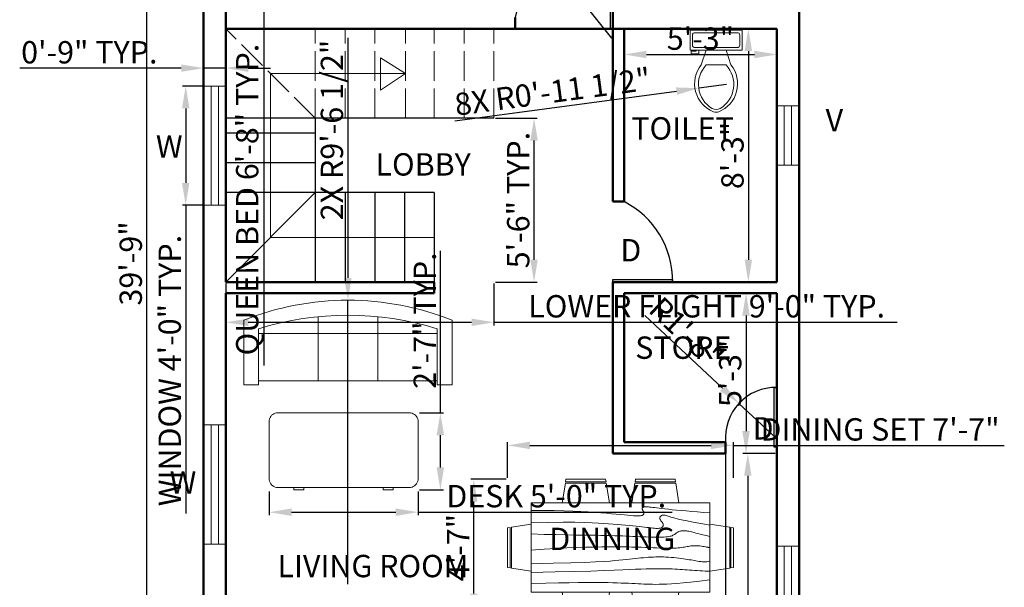
# Model space of a CAD drawing. Units: inches. Extents: x 1802 to 2621, y 1038 to 1686.
# Tile 2 of 5: x 1802 to 2198, y 1223 to 1452. Entities that reach past the tile are written whole.
import ezdxf

# ---------------------------------------------------------------- set-up
doc = ezdxf.new("R2010")
doc.units = ezdxf.units.IN
doc.linetypes.add('ACAD_ISO02W100', pattern=[15, 12, -3])
for name, color, linetype, lineweight in [('A-ANNO-DIMS', 2, 'Continuous', 18), ('A-ANNO-SYMB', 7, 'Continuous', 18), ('A-ANNO-TEXT', 7, 'Continuous', 18), ('A-AREA-IDEN', 7, 'Continuous', 25), ('A-DOOR', 3, 'Continuous', 25), ('A-FLOR-FIXT', 9, 'Continuous', 18), ('A-FLOR-STRS', 7, 'Continuous', 25), ('A-FLOR-STRS-OVHD', 8, 'ACAD_ISO02W100', 18), ('A-FURN', 8, 'Continuous', 18), ('A-GLAZ', 4, 'Continuous', 18), ('A-WALL', 7, 'Continuous', 50)]:
    doc.layers.add(name, color=color, linetype=linetype, lineweight=lineweight)
doc.styles.get("Standard").update_dxf_attribs({"font": 'arial.ttf'})
doc.dimstyles.new('ISO-25', dxfattribs={"dimtxt": 9, "dimasz": 9, "dimexe": 1.25, "dimexo": 0.625, "dimtad": 1, "dimdec": 1, "dimrnd": 9, "dimlunit": 3, "dimtxsty": 'Standard', "dimcen": 2.5, "dimadec": 0, "dimazin": 0, "dimtfac": 1, "dimtdec": 1, "dimtmove": 0, "dimatfit": 3, "dimfxl": 1, "dimarcsym": 0})

# ---------------------------------------------------------------- blocks, each defined once
blk = doc.blocks.new('*D4')
at = {"layer": 'A-ANNO-DIMS', "color": 0, "lineweight": -2, "transparency": 16777216}
for p, q in [((1875.1, 1593.56), (1851.51, 1593.56)), ((1852.76, 1584.56), (1852.76, 1122.56)), ((1875.1, 1113.56), (1851.51, 1113.56))]:
    blk.add_line(p, q, dxfattribs=at)
at = {"layer": 'A-ANNO-DIMS', "color": 0, "transparency": 16777216}
for points in [[(1851.26, 1584.56), (1854.26, 1584.56), (1852.76, 1593.56)], [(1851.26, 1122.56), (1854.26, 1122.56), (1852.76, 1113.56)]]:
    blk.add_solid(points, dxfattribs=at)
at = {"layer": 'Defpoints', "color": 0, "transparency": 16777216}
for p in [(1875.73, 1593.56), (1852.76, 1113.56), (1875.73, 1113.56)]:
    blk.add_point(p, dxfattribs=at)
at = {"layer": 'A-ANNO-DIMS', "color": 0, "transparency": 16777216, "insert": (1847.54, 1353.56), "char_height": 9, "attachment_point": 5, "rotation": 90}
blk.add_mtext('39\'-9"', dxfattribs=at)
blk = doc.blocks.new('*D6')
at = {"layer": 'A-ANNO-DIMS', "color": 0, "lineweight": -2, "transparency": 16777216}
for p, q in [((2106.1, 1448.06), (2094.04, 1448.06)), ((2095.29, 1439.06), (2095.29, 1355.06)), ((2106.1, 1346.06), (2094.04, 1346.06))]:
    blk.add_line(p, q, dxfattribs=at)
at = {"layer": 'A-ANNO-DIMS', "color": 0, "transparency": 16777216}
for points in [[(2093.79, 1439.06), (2096.79, 1439.06), (2095.29, 1448.06)], [(2093.79, 1355.06), (2096.79, 1355.06), (2095.29, 1346.06)]]:
    blk.add_solid(points, dxfattribs=at)
at = {"layer": 'Defpoints', "color": 0, "transparency": 16777216}
for p in [(2106.73, 1448.06), (2095.29, 1346.06), (2106.73, 1346.06)]:
    blk.add_point(p, dxfattribs=at)
at = {"layer": 'A-ANNO-DIMS', "color": 0, "transparency": 16777216, "insert": (2090.06, 1397.06), "char_height": 9, "attachment_point": 5, "rotation": 90}
blk.add_mtext('8\'-3"', dxfattribs=at)
blk = doc.blocks.new('*D7')
at = {"layer": 'A-ANNO-DIMS', "color": 0, "lineweight": -2, "transparency": 16777216}
for p, q in [((2106.1, 1341.56), (2093.11, 1341.56)), ((2094.36, 1332.56), (2094.36, 1286.06)), ((2106.1, 1277.06), (2093.11, 1277.06))]:
    blk.add_line(p, q, dxfattribs=at)
at = {"layer": 'A-ANNO-DIMS', "color": 0, "transparency": 16777216}
for points in [[(2092.86, 1332.56), (2095.86, 1332.56), (2094.36, 1341.56)], [(2092.86, 1286.06), (2095.86, 1286.06), (2094.36, 1277.06)]]:
    blk.add_solid(points, dxfattribs=at)
at = {"layer": 'Defpoints', "color": 0, "transparency": 16777216}
for p in [(2106.73, 1341.56), (2094.36, 1277.06), (2106.73, 1277.06)]:
    blk.add_point(p, dxfattribs=at)
at = {"layer": 'A-ANNO-DIMS', "color": 0, "transparency": 16777216, "insert": (2089.14, 1309.31), "char_height": 9, "attachment_point": 5, "rotation": 90}
blk.add_mtext('5\'-3"', dxfattribs=at)
blk = doc.blocks.new('*D8')
at = {"layer": 'A-ANNO-DIMS', "color": 0, "lineweight": -2, "transparency": 16777216}
for p, q in [((2106.1, 1277.06), (2093.83, 1277.06)), ((2095.08, 1268.06), (2095.08, 1131.56)), ((2106.1, 1122.56), (2093.83, 1122.56))]:
    blk.add_line(p, q, dxfattribs=at)
at = {"layer": 'A-ANNO-DIMS', "color": 0, "transparency": 16777216}
for points in [[(2093.58, 1268.06), (2096.58, 1268.06), (2095.08, 1277.06)], [(2093.58, 1131.56), (2096.58, 1131.56), (2095.08, 1122.56)]]:
    blk.add_solid(points, dxfattribs=at)
at = {"layer": 'Defpoints', "color": 0, "transparency": 16777216}
for p in [(2106.73, 1277.06), (2095.08, 1122.56), (2106.73, 1122.56)]:
    blk.add_point(p, dxfattribs=at)
at = {"layer": 'A-ANNO-DIMS', "color": 0, "transparency": 16777216, "insert": (2089.86, 1199.81), "char_height": 9, "attachment_point": 5, "rotation": 90}
blk.add_mtext('12\'-9"', dxfattribs=at)
blk = doc.blocks.new('*D11')
at = {"layer": 'A-ANNO-DIMS', "color": 0, "lineweight": -2, "transparency": 16777216}
for p, q in [((2045.23, 1447.43), (2045.23, 1436.45)), ((2106.73, 1447.43), (2106.73, 1436.45)), ((2054.23, 1437.7), (2097.73, 1437.7))]:
    blk.add_line(p, q, dxfattribs=at)
at = {"layer": 'A-ANNO-DIMS', "color": 0, "transparency": 16777216}
for points in [[(2054.23, 1439.2), (2054.23, 1436.2), (2045.23, 1437.7)], [(2097.73, 1439.2), (2097.73, 1436.2), (2106.73, 1437.7)]]:
    blk.add_solid(points, dxfattribs=at)
at = {"layer": 'Defpoints', "color": 0, "transparency": 16777216}
for p in [(2045.23, 1448.06), (2106.73, 1448.06), (2106.73, 1437.7)]:
    blk.add_point(p, dxfattribs=at)
at = {"layer": 'A-ANNO-DIMS', "color": 0, "transparency": 16777216, "insert": (2075.98, 1442.92), "char_height": 9, "attachment_point": 5}
blk.add_mtext('5\'-3"', dxfattribs=at)
blk = doc.blocks.new('Dining Set - 36 x 72 in.')
for p, q in [((-22.2343, 26.00059), (-23.4847, 17.99762)), ((-22.2304, 26), (-5.7608, 26)), ((-22, 27.5), (-22.1562, 26.50042)), ((-5.8416, 26.5), (-22.1534, 26.5)), ((-22, 27.5), (-6, 27.5)), ((-5.8437, 26.49966), (-6, 27.5)), ((-4.5152, 17.99762), (-5.7655, 25.99926)), ((5.7657, 26.00059), (4.5153, 17.99762)), ((5.7696, 26), (22.2392, 26)), ((6, 27.5), (5.8438, 26.50042)), ((22.1584, 26.5), (5.8466, 26.5)), ((6, 27.5), (22, 27.5)), ((22.1563, 26.49966), (22, 27.5)), ((23.4848, 17.99762), (22.2345, 25.99926)), ((36, 18), (-36, 18)), ((-36, 18), (-36, -18)), ((36, -18), (36, 18)), ((-45.5, 8), (-44.5004, 8.15617)), ((-45.5, 8), (-45.5, -8)), ((-44.5, -8.15843), (-44.5, 8.15338)), ((-44.0006, 8.23428), (-35.9976, 9.48474)), ((-44, 8.23041), (-44, -8.23915)), ((44.0006, 8.23428), (35.9976, 9.48474)), ((44, 8.23041), (44, -8.23915)), ((44.5, -8.15843), (44.5, 8.15338)), ((45.5, 8), (44.5005, 8.15617)), ((45.5, 8), (45.5, -8)), ((-44.4997, -8.15631), (-45.5, -8)), ((-35.9976, -9.48476), (-43.9993, -8.2345)), ((35.9976, -9.48476), (43.9993, -8.2345)), ((44.4997, -8.15631), (45.5, -8)), ((-36, -18), (36, -18)), ((-22.2343, -26.0006), (-23.4847, -17.99762)), ((-4.5152, -17.99762), (-5.7655, -25.99928)), ((5.7657, -26.0006), (4.5153, -17.99762)), ((23.4848, -17.99762), (22.2345, -25.99928)), ((-22.2304, -26), (-5.7608, -26)), ((-22, -27.5), (-22.1562, -26.50044)), ((-5.8416, -26.5), (-22.1534, -26.5)), ((-22, -27.5), (-6, -27.5)), ((-5.8437, -26.49967), (-6, -27.5)), ((5.7696, -26), (22.2392, -26)), ((6, -27.5), (5.8438, -26.50044)), ((22.1584, -26.5), (5.8466, -26.5)), ((6, -27.5), (22, -27.5)), ((22.1563, -26.49967), (22, -27.5))]:
    blk.add_line(p, q)
for points in [[(-36, 15), (-31.1772, 14.97754), (-26.8079, 14.91406), (-22.8538, 14.81543), (-19.276, 14.6875), (-16.0362, 14.53613), (-13.0957, 14.36718), (-10.4159, 14.18652), (-7.9583, 14), (-5.6904, 13.81315), (-3.6035, 13.63021), (-1.6954, 13.45508), (0.0365, 13.29166), (1.5945, 13.14388), (2.9811, 13.01562), (4.1988, 12.9108), (5.25, 12.83333), (6.1393, 12.78613), (6.8802, 12.76823), (7.4883, 12.77767), (7.9792, 12.8125), (8.3685, 12.87077), (8.6719, 12.95052), (8.9049, 13.0498), (9.0833, 13.16666), (9.2205, 13.29899), (9.3216, 13.44401), (9.3895, 13.59879), (9.4271, 13.76041), (9.4373, 13.92594), (9.4232, 14.09245), (9.3875, 14.257), (9.3333, 14.41666), (9.2638, 14.56917), (9.1836, 14.71484), (9.0975, 14.85465), (9.0104, 14.98958), (8.9272, 15.1206), (8.8529, 15.2487), (8.7922, 15.37483), (8.75, 15.5), (8.7305, 15.62467), (8.7344, 15.74739), (8.7617, 15.86621), (8.8125, 15.97916), (8.8867, 16.08431), (8.9844, 16.17968), (9.1055, 16.26334), (9.25, 16.33333), (9.4189, 16.38802), (9.6172, 16.42708), (9.8506, 16.45052), (10.125, 16.45833), (10.4463, 16.45052), (10.8203, 16.42708), (11.2529, 16.38802), (11.75, 16.33333), (12.3184, 16.26318), (12.9694, 16.17838), (13.7151, 16.07991), (14.5677, 15.96875), (15.5395, 15.84586), (16.6426, 15.71224), (17.8893, 15.56884), (19.2917, 15.41666), (20.859, 15.25667), (22.5879, 15.08984), (24.4721, 14.91715), (26.5052, 14.73958), (28.6809, 14.5581), (30.9929, 14.3737), (33.4347, 14.18733), (36, 14)], [(-36, 10), (-28.9766, 10.14274), (-23.1725, 10.20442), (-18.4241, 10.19775), (-14.5677, 10.13541), (-11.4399, 10.03011), (-8.877, 9.89453), (-6.7154, 9.74137), (-4.7917, 9.58333), (-2.9698, 9.43082), (-1.2246, 9.28515), (0.4415, 9.14534), (2.026, 9.01041), (3.5266, 8.87939), (4.9408, 8.7513), (6.266, 8.62516), (7.5, 8.5), (8.6411, 8.37549), (9.6914, 8.2539), (10.6538, 8.13818), (11.5312, 8.03125), (12.3267, 7.93603), (13.043, 7.85547), (13.6831, 7.79248), (14.25, 7.75), (14.7471, 7.7303), (15.1797, 7.73307), (15.5537, 7.75732), (15.875, 7.80208), (16.1494, 7.86637), (16.3828, 7.94922), (16.5811, 8.04964), (16.75, 8.16666), (16.8944, 8.29915), (17.0143, 8.44531), (17.1089, 8.60319), (17.1771, 8.77083), (17.218, 8.94629), (17.2305, 9.1276), (17.2137, 9.31282), (17.1667, 9.5), (17.0895, 9.6875), (16.987, 9.875), (16.8649, 10.0625), (16.7292, 10.25), (16.5856, 10.4375), (16.4401, 10.625), (16.2985, 10.8125), (16.1667, 11), (16.05, 11.18733), (15.9518, 11.3737), (15.8752, 11.5581), (15.8229, 11.73958), (15.798, 11.91715), (15.8034, 12.08984), (15.842, 12.25667), (15.9167, 12.41666), (16.0295, 12.56836), (16.1784, 12.70833), (16.3605, 12.83268), (16.5729, 12.9375), (16.8127, 13.01888), (17.0768, 13.07291), (17.3625, 13.0957), (17.6667, 13.08333), (17.9894, 13.03312), (18.3418, 12.94726), (18.7382, 12.82918), (19.1927, 12.68229), (19.7195, 12.51001), (20.3327, 12.31575), (21.0465, 12.10294), (21.875, 11.875), (22.8357, 11.63354), (23.959, 11.37304), (25.2786, 11.08618), (26.8282, 10.76562), (28.6414, 10.40405), (30.752, 9.99414), (33.1936, 9.52856), (36, 9)], [(-36, 5.5), (-30.7157, 5.3348), (-26.069, 5.20963), (-21.9946, 5.11767), (-18.4271, 5.05208), (-15.3009, 5.00602), (-12.5508, 4.97265), (-10.1112, 4.94515), (-7.9167, 4.91666), (-5.909, 4.88167), (-4.0586, 4.83984), (-2.3429, 4.79215), (-0.7396, 4.73958), (0.7739, 4.6831), (2.22, 4.6237), (3.6213, 4.56233), (5, 4.5), (6.373, 4.43782), (7.7344, 4.3776), (9.0723, 4.32129), (10.375, 4.27083), (11.6309, 4.22819), (12.8281, 4.19531), (13.9551, 4.17415), (15, 4.16666), (15.954, 4.17448), (16.819, 4.19791), (17.6001, 4.23698), (18.3021, 4.29166), (18.9299, 4.36198), (19.4883, 4.44791), (19.9823, 4.54948), (20.4167, 4.66666), (20.7969, 4.79899), (21.1302, 4.94401), (21.4245, 5.09879), (21.6875, 5.26041), (21.9271, 5.42594), (22.1511, 5.59245), (22.3672, 5.757), (22.5834, 5.91666), (22.8065, 6.06868), (23.0404, 6.21093), (23.2879, 6.34147), (23.5521, 6.45833), (23.8358, 6.55957), (24.142, 6.64323), (24.4735, 6.70735), (24.8334, 6.75), (25.2235, 6.76969), (25.642, 6.76692), (26.0858, 6.74267), (26.5521, 6.69791), (27.0379, 6.63362), (27.5404, 6.55078), (28.0565, 6.45036), (28.5834, 6.33333), (29.1242, 6.19987), (29.7071, 6.04687), (30.3661, 5.87044), (31.1354, 5.66666), (32.0493, 5.43164), (33.142, 5.16146), (34.4475, 4.85221), (36, 4.5)], [(-36, -1), (-30.7915, -0.6591), (-26.0195, -0.38216), (-21.6519, -0.16284), (-17.6563, 0.00521), (-14.0005, 0.12833), (-10.6523, 0.21289), (-7.5796, 0.26522), (-4.75, 0.29166), (-2.134, 0.29793), (0.2878, 0.28711), (2.5317, 0.26163), (4.6146, 0.22396), (6.5529, 0.17651), (8.3633, 0.12174), (10.0623, 0.06209), (11.6667, 0), (13.1899, -0.06201), (14.6341, -0.1211), (15.9982, -0.17432), (17.2813, -0.21875), (18.4823, -0.25147), (19.6003, -0.26953), (20.6343, -0.27002), (21.5834, -0.25), (22.4481, -0.20768), (23.2357, -0.14584), (23.9549, -0.06836), (24.6146, 0.02083), (25.2235, 0.11784), (25.7904, 0.21875), (26.3241, 0.31966), (26.8334, 0.41666), (27.3265, 0.50618), (27.8099, 0.58593), (28.2894, 0.65397), (28.7709, 0.70833), (29.2601, 0.74707), (29.763, 0.76823), (30.2855, 0.76985), (30.8334, 0.75), (31.4088, 0.70784), (31.9994, 0.64713), (32.589, 0.57275), (33.1615, 0.48958), (33.7008, 0.4025), (34.1908, 0.3164), (34.6153, 0.23616), (34.9584, 0.16666), (35.2099, 0.11165), (35.3848, 0.07031), (35.504, 0.04069), (35.5886, 0.02083), (35.6594, 0.00879), (35.7377, 0.0026), (35.8442, 0.00032), (36, 0)], [(-36, -6.5), (-27.1843, -6.31267), (-20.084, -6.1263), (-14.469, -5.9419), (-10.1094, -5.76042), (-6.7752, -5.58285), (-4.2363, -5.41016), (-2.2629, -5.24333), (-0.625, -5.08334), (0.8708, -4.93099), (2.2715, -4.78646), (3.5872, -4.64974), (4.8281, -4.52084), (6.0046, -4.39974), (7.127, -4.28646), (8.2053, -4.18099), (9.25, -4.08334), (10.2705, -3.99382), (11.2734, -3.91407), (12.2647, -3.84603), (13.25, -3.79167), (14.2354, -3.75293), (15.2266, -3.73177), (16.2295, -3.73015), (17.25, -3.75), (18.2912, -3.79248), (19.3451, -3.85547), (20.4009, -3.93604), (21.4479, -4.03125), (22.4754, -4.13819), (23.4727, -4.25391), (24.4289, -4.37549), (25.3334, -4.5), (26.1785, -4.62492), (26.9694, -4.74935), (27.7145, -4.87281), (28.4219, -4.99479), (29.1, -5.11483), (29.7572, -5.23242), (30.4016, -5.34709), (31.0417, -5.45834), (31.6837, -5.56437), (32.3262, -5.65821), (32.9658, -5.73153), (33.599, -5.77604), (34.2224, -5.78345), (34.8327, -5.74545), (35.4264, -5.65373), (36, -5.5)], [(-36, -10), (-26.4022, -9.81299), (-18.4675, -9.62891), (-11.9839, -9.45069), (-6.7396, -9.28125), (-2.5226, -9.12354), (0.8789, -8.98047), (3.6769, -8.85498), (6.0833, -8.75), (8.2767, -8.66765), (10.3021, -8.60677), (12.1712, -8.56543), (13.8958, -8.54167), (15.4876, -8.53353), (16.9583, -8.53907), (18.3197, -8.55632), (19.5834, -8.58334), (20.7616, -8.61841), (21.8685, -8.66081), (22.9188, -8.71004), (23.9271, -8.76563), (24.9081, -8.82707), (25.8763, -8.89388), (26.8465, -8.96558), (27.8334, -9.04167), (28.8474, -9.12118), (29.8828, -9.20117), (30.93, -9.27824), (31.9792, -9.34896), (33.0205, -9.40991), (34.0443, -9.45768), (35.0407, -9.48885), (36, -9.5)], [(-36, -14.5), (-30.0881, -14.33513), (-25.0332, -14.21224), (-20.7312, -14.12647), (-17.0781, -14.07292), (-13.97, -14.04671), (-11.3027, -14.04297), (-8.9724, -14.05681), (-6.875, -14.08334), (-4.9224, -14.11833), (-3.0905, -14.16016), (-1.3709, -14.20785), (0.2448, -14.26042), (1.7647, -14.3169), (3.1973, -14.3763), (4.5507, -14.43767), (5.8333, -14.5), (7.0554, -14.5621), (8.235, -14.62175), (9.3922, -14.67652), (10.5469, -14.72396), (11.7192, -14.76164), (12.929, -14.78711), (14.1965, -14.79794), (15.5417, -14.79167), (16.9933, -14.76424), (18.6152, -14.70508), (20.4804, -14.60197), (22.6615, -14.44271), (25.2312, -14.21509), (28.2624, -13.9069), (31.8277, -13.50594), (36, -13)]]:
    blk.add_lwpolyline(points)
blk = doc.blocks.new('Toilet - top')
for p, q in [((9.5, -6), (9.5, -2)), ((-10, -8.5), (-8, -8.5)), ((-10, -9.5), (-10, -8.5)), ((-7, -9.5), (-10, -9.5)), ((-8, -8.5), (-8, -8)), ((-7, -8), (-7, -9.5)), ((-4, -8), (-6, -14)), ((4, -8), (6, -14)), ((4, -14), (-4, -14))]:
    blk.add_line(p, q)
blk.add_lwpolyline([(10.5, -8), (10.5, 0), (-10.5, 0), (-10.5, -8)], close=True)
for points in [[(-9.5, -2), (-9.5, -6)], [(8.5, -1), (-8.5, -1)], [(-8.5, -7), (8.5, -7)]]:
    blk.add_lwpolyline(points)
for centre, radius, start, end in [((-8.62, -1.88), 0.884, 81.8699, 188.1301), ((8.62, -1.88), 0.884, 351.8699, 98.1301), ((-8.62, -6.12), 0.884, 171.8699, 278.1301), ((8.62, -6.12), 0.884, 261.8699, 8.1301), ((3.52, -21.58), 12.17, 141.4691, 247.9714), ((4.2, -21.82), 11.33, 136.3677, 238.9468), ((-3.52, -21.58), 12.17, 292.0284, 38.5307), ((-4.2, -21.82), 11.33, 301.053, 43.6321), ((0, -27.88), 4, 245.7318, 294.2682), ((0, -29), 4, 254.8605, 285.1395)]:
    blk.add_arc(centre, radius, start, end)
blk = doc.blocks.new('Sofa - Roundback 7 ft.')
for p, q in [((-12.00002, -32.4421), (-12.00003, -6.5971)), ((11.99997, -32.4421), (11.99998, -6.5971)), ((-36.000027, -34), (-36.000027, -11.4696)), ((35.99998, -34), (35.99998, -11.4696)), ((-35.999844, -13.3819), (35.9998, -13.3819)), ((-36.000027, -32.4421), (35.99998, -32.4421))]:
    blk.add_line(p, q)
for points in [[(-36.000027, -34), (-42.000027, -34), (-42.000027, -8)], [(41.99998, -8), (41.99998, -34), (35.99998, -34)]]:
    blk.add_lwpolyline(points)
for centre, radius, start, end in [((0, -114.25), 114.25, 68.43141, 111.5686), ((-0.00001, -127.1968), 121.1968, 72.72033, 107.2797)]:
    blk.add_arc(centre, radius, start, end)
blk = doc.blocks.new('Desk - 30 x 60 in.')
for p, q in [((-26.999995, 0), (26.999995, 0)), ((-29.999995, -27), (-29.999995, -3)), ((29.999995, -3), (29.999995, -27)), ((26.999995, -30), (-26.999995, -30)), ((-20.000005, -30), (-20.000005, -31)), ((-20.000005, -31), (-16.000005, -31)), ((-16.000005, -31), (-16.000005, -30)), ((15.999995, -31), (15.999995, -30)), ((19.999995, -31), (15.999995, -31)), ((19.999995, -30), (19.999995, -31))]:
    blk.add_line(p, q)
for centre, start, end in [((-26.499995, -3.5), 98.1301, 171.8699), ((26.499995, -3.5), 8.130102, 81.8699), ((-26.499995, -26.5), 188.1301, 261.8699), ((26.499995, -26.5), 278.1301, 351.8699)]:
    blk.add_arc(centre, 3.535534, start, end)
blk = doc.blocks.new('WIN-48IN')
for p, q in [((9, 48), (0, 48)), ((3, 48), (3, 0)), ((6, 48), (6, 0)), ((9, 0), (0, 0))]:
    blk.add_line(p, q)
blk = doc.blocks.new('VENT-24IN')
for p, q in [((0, 24), (9, 24)), ((3, 0), (3, 24)), ((6, 0), (6, 24)), ((0, 0), (9, 0))]:
    blk.add_line(p, q)
blk = doc.blocks.new('DOOR-BEDROOM-36IN')
for p, q in [((38.47, 0), (38.47, 36)), ((38.47, 36), (39.47, 36)), ((39.47, 0), (38.47, 0))]:
    blk.add_line(p, q)
blk.add_arc((38.97, -3.86), 39.86, 89.2813, 167.8967)
blk = doc.blocks.new('DOOR-BATH-LOBBY-24IN')
for p, q in [((0, 0), (0, 1)), ((0, 1), (24, 1)), ((24, 1), (24, 0))]:
    blk.add_line(p, q)
blk.add_arc((-11.84, 0.5), 35.84, 359.2007, 62.8783)
blk = doc.blocks.new('STAIR-DIRECTION-U')
for p, q in [((44.37, 59.29), (44.37, 72.31)), ((44.37, 72.31), (54.34, 66)), ((0, 0), (0, 66)), ((0, 66), (54.34, 66)), ((54.34, 66), (44.37, 59.29)), ((66, 0), (0, 0))]:
    blk.add_line(p, q)
blk = doc.blocks.new('STAIR-WINDER-UPPER-TREADS')
for p, q in [((36, 0), (0, 36)), ((36, 0), (36, 36)), ((48, 0), (48, 36)), ((60, 0), (60, 36)), ((72.34, 0), (72.34, 36)), ((84, 0), (84, 36)), ((96, 0), (96, 36)), ((108, 0), (108, 36))]:
    blk.add_line(p, q)
blk = doc.blocks.new('STAIR-WINDER-VISIBLE')
for p, q in [((108, 66), (0, 66)), ((36, 66), (36, 0)), ((36, 60), (0, 60)), ((36, 48), (0, 48)), ((84, 36), (0, 36)), ((36, 36), (0, 0)), ((48, 36), (48, 0)), ((60, 36), (60, 0)), ((72, 36), (72, 0)), ((84, 36), (84, 0))]:
    blk.add_line(p, q)
blk = doc.blocks.new('*D37')
at = {"layer": 'A-ANNO-DIMS', "color": 0, "lineweight": -2, "transparency": 16777216}
for p, q in [((1875.1, 1425), (1867.28, 1425)), ((1868.53, 1416), (1868.53, 1386)), ((1875.1, 1377), (1867.28, 1377)), ((1868.53, 1377), (1868.53, 1252.86))]:
    blk.add_line(p, q, dxfattribs=at)
at = {"layer": 'A-ANNO-DIMS', "color": 0, "transparency": 16777216}
for points in [[(1867.03, 1416), (1870.03, 1416), (1868.53, 1425)], [(1867.03, 1386), (1870.03, 1386), (1868.53, 1377)]]:
    blk.add_solid(points, dxfattribs=at)
at = {"layer": 'Defpoints', "color": 0, "transparency": 16777216}
for p in [(1875.73, 1425), (1868.53, 1377), (1875.73, 1377)]:
    blk.add_point(p, dxfattribs=at)
at = {"layer": 'A-ANNO-DIMS', "color": 0, "transparency": 16777216, "insert": (1863.25, 1310.43), "char_height": 9, "attachment_point": 5, "rotation": 90}
blk.add_mtext('WINDOW 4\'-0" TYP.', dxfattribs=at)
blk = doc.blocks.new('*D38')
at = {"layer": 'A-ANNO-DIMS', "color": 0, "lineweight": -2, "transparency": 16777216}
for p, q in [((1875.73, 1425.62), (1875.73, 1433.45)), ((1884.73, 1425.62), (1884.73, 1433.45)), ((1866.73, 1432.2), (1801.62, 1432.2)), ((1884.73, 1432.2), (1875.73, 1432.2)), ((1893.73, 1432.2), (1902.73, 1432.2))]:
    blk.add_line(p, q, dxfattribs=at)
at = {"layer": 'A-ANNO-DIMS', "color": 0, "transparency": 16777216}
for points in [[(1866.73, 1433.7), (1866.73, 1430.7), (1875.73, 1432.2)], [(1893.73, 1433.7), (1893.73, 1430.7), (1884.73, 1432.2)]]:
    blk.add_solid(points, dxfattribs=at)
at = {"layer": 'Defpoints', "color": 0, "transparency": 16777216}
for p in [(1875.73, 1432.2), (1875.73, 1425), (1884.73, 1425)]:
    blk.add_point(p, dxfattribs=at)
at = {"layer": 'A-ANNO-DIMS', "color": 0, "transparency": 16777216, "insert": (1829.68, 1437.42), "char_height": 9, "attachment_point": 5}
blk.add_mtext('0\'-9" TYP.', dxfattribs=at)
blk = doc.blocks.new('*D43')
at = {"layer": 'A-ANNO-DIMS', "color": 0, "lineweight": -2, "transparency": 16777216}
for p, q in [((1911.42, 1535.09), (1898.79, 1535.09)), ((1900.04, 1526.09), (1900.04, 1464.09)), ((1911.42, 1455.09), (1898.79, 1455.09)), ((1900.04, 1455.09), (1900.04, 1312.45))]:
    blk.add_line(p, q, dxfattribs=at)
at = {"layer": 'A-ANNO-DIMS', "color": 0, "transparency": 16777216}
for points in [[(1898.54, 1526.09), (1901.54, 1526.09), (1900.04, 1535.09)], [(1898.54, 1464.09), (1901.54, 1464.09), (1900.04, 1455.09)]]:
    blk.add_solid(points, dxfattribs=at)
at = {"layer": 'Defpoints', "color": 0, "transparency": 16777216}
for p in [(1912.04, 1535.09), (1900.04, 1455.09), (1912.04, 1455.09)]:
    blk.add_point(p, dxfattribs=at)
at = {"layer": 'A-ANNO-DIMS', "color": 0, "transparency": 16777216, "insert": (1894.49, 1379.27), "char_height": 9, "attachment_point": 5, "rotation": 90}
blk.add_mtext('QUEEN BED 6\'-8" TYP.', dxfattribs=at)
blk = doc.blocks.new('*D47')
at = {"layer": 'A-ANNO-DIMS', "color": 0, "lineweight": -2, "transparency": 16777216}
for p, q in [((1902.17, 1261.78), (1902.17, 1252.16)), ((1962.17, 1261.78), (1962.17, 1252.16)), ((1911.17, 1253.41), (1953.17, 1253.41)), ((1962.17, 1253.41), (2064.56, 1253.41))]:
    blk.add_line(p, q, dxfattribs=at)
at = {"layer": 'A-ANNO-DIMS', "color": 0, "transparency": 16777216}
for points in [[(1911.17, 1254.91), (1911.17, 1251.91), (1902.17, 1253.41)], [(1953.17, 1254.91), (1953.17, 1251.91), (1962.17, 1253.41)]]:
    blk.add_solid(points, dxfattribs=at)
at = {"layer": 'Defpoints', "color": 0, "transparency": 16777216}
for p in [(1902.17, 1262.41), (1962.17, 1262.41), (1962.17, 1253.41)]:
    blk.add_point(p, dxfattribs=at)
at = {"layer": 'A-ANNO-DIMS', "color": 0, "transparency": 16777216, "insert": (2017.87, 1258.69), "char_height": 9, "attachment_point": 5}
blk.add_mtext('DESK 5\'-0" TYP.', dxfattribs=at)
blk = doc.blocks.new('*D48')
at = {"layer": 'A-ANNO-DIMS', "color": 0, "lineweight": -2, "transparency": 16777216}
for p, q in [((1971.17, 1293.41), (1971.17, 1358.67)), ((1962.8, 1293.41), (1972.42, 1293.41)), ((1971.17, 1271.41), (1971.17, 1284.41)), ((1962.8, 1262.41), (1972.42, 1262.41))]:
    blk.add_line(p, q, dxfattribs=at)
at = {"layer": 'A-ANNO-DIMS', "color": 0, "transparency": 16777216}
for points in [[(1969.67, 1284.41), (1972.67, 1284.41), (1971.17, 1293.41)], [(1969.67, 1271.41), (1972.67, 1271.41), (1971.17, 1262.41)]]:
    blk.add_solid(points, dxfattribs=at)
at = {"layer": 'Defpoints', "color": 0, "transparency": 16777216}
for p in [(1962.17, 1293.41), (1971.17, 1293.41), (1962.17, 1262.41)]:
    blk.add_point(p, dxfattribs=at)
at = {"layer": 'A-ANNO-DIMS', "color": 0, "transparency": 16777216, "insert": (1966.03, 1330.54), "char_height": 9, "attachment_point": 5, "rotation": 90}
blk.add_mtext('2\'-7" TYP.', dxfattribs=at)
blk = doc.blocks.new('*D55')
at = {"layer": 'A-ANNO-DIMS', "color": 0, "lineweight": -2, "transparency": 16777216}
for p, q in [((1884.73, 1345.43), (1884.73, 1328.61)), ((1992.73, 1345.43), (1992.73, 1328.61)), ((1893.73, 1329.86), (1983.73, 1329.86)), ((1992.73, 1329.86), (2155.24, 1329.86))]:
    blk.add_line(p, q, dxfattribs=at)
at = {"layer": 'A-ANNO-DIMS', "color": 0, "transparency": 16777216}
for points in [[(1893.73, 1331.36), (1893.73, 1328.36), (1884.73, 1329.86)], [(1983.73, 1331.36), (1983.73, 1328.36), (1992.73, 1329.86)]]:
    blk.add_solid(points, dxfattribs=at)
at = {"layer": 'Defpoints', "color": 0, "transparency": 16777216}
for p in [(1884.73, 1346.06), (1992.73, 1346.06), (1992.73, 1329.86)]:
    blk.add_point(p, dxfattribs=at)
at = {"layer": 'A-ANNO-DIMS', "color": 0, "transparency": 16777216, "insert": (2078.48, 1335.14), "char_height": 9, "attachment_point": 5}
blk.add_mtext('LOWER FLIGHT 9\'-0" TYP.', dxfattribs=at)
blk = doc.blocks.new('*D56')
at = {"layer": 'A-ANNO-DIMS', "color": 0, "lineweight": -2, "transparency": 16777216}
for p, q in [((1993.35, 1412.06), (2010.18, 1412.06)), ((2008.93, 1355.06), (2008.93, 1403.06)), ((1993.35, 1346.06), (2010.18, 1346.06))]:
    blk.add_line(p, q, dxfattribs=at)
at = {"layer": 'A-ANNO-DIMS', "color": 0, "transparency": 16777216}
for points in [[(2007.43, 1403.06), (2010.43, 1403.06), (2008.93, 1412.06)], [(2007.43, 1355.06), (2010.43, 1355.06), (2008.93, 1346.06)]]:
    blk.add_solid(points, dxfattribs=at)
at = {"layer": 'Defpoints', "color": 0, "transparency": 16777216}
for p in [(1992.73, 1412.06), (2008.93, 1412.06), (1992.73, 1346.06)]:
    blk.add_point(p, dxfattribs=at)
at = {"layer": 'A-ANNO-DIMS', "color": 0, "transparency": 16777216, "insert": (2003.71, 1379.06), "char_height": 9, "attachment_point": 5, "rotation": 90}
blk.add_mtext('5\'-6" TYP.', dxfattribs=at)
blk = doc.blocks.new('*D59')
at = {"layer": 'A-ANNO-DIMS', "color": 0, "lineweight": -2, "transparency": 16777216}
for p, q in [((1998.28, 1267.27), (1998.28, 1281.55)), ((2007.28, 1280.3), (2080.28, 1280.3)), ((2089.28, 1267.27), (2089.28, 1281.55)), ((2089.28, 1280.3), (2198.45, 1280.3))]:
    blk.add_line(p, q, dxfattribs=at)
at = {"layer": 'A-ANNO-DIMS', "color": 0, "transparency": 16777216}
for points in [[(2007.28, 1281.8), (2007.28, 1278.8), (1998.28, 1280.3)], [(2080.28, 1281.8), (2080.28, 1278.8), (2089.28, 1280.3)]]:
    blk.add_solid(points, dxfattribs=at)
at = {"layer": 'Defpoints', "color": 0, "transparency": 16777216}
for p in [(2089.28, 1280.3), (1998.28, 1266.65), (2089.28, 1266.65)]:
    blk.add_point(p, dxfattribs=at)
at = {"layer": 'A-ANNO-DIMS', "color": 0, "transparency": 16777216, "insert": (2148.37, 1285.58), "char_height": 9, "attachment_point": 5}
blk.add_mtext('DINING SET 7\'-7"', dxfattribs=at)
blk = doc.blocks.new('*D60')
at = {"layer": 'A-ANNO-DIMS', "color": 0, "lineweight": -2, "transparency": 16777216}
for p, q in [((1997.66, 1266.65), (1983.38, 1266.65)), ((1984.63, 1220.65), (1984.63, 1257.65)), ((1997.66, 1211.65), (1983.38, 1211.65))]:
    blk.add_line(p, q, dxfattribs=at)
at = {"layer": 'A-ANNO-DIMS', "color": 0, "transparency": 16777216}
for points in [[(1983.13, 1257.65), (1986.13, 1257.65), (1984.63, 1266.65)], [(1983.13, 1220.65), (1986.13, 1220.65), (1984.63, 1211.65)]]:
    blk.add_solid(points, dxfattribs=at)
at = {"layer": 'Defpoints', "color": 0, "transparency": 16777216}
for p in [(1984.63, 1266.65), (1998.28, 1266.65), (1998.28, 1211.65)]:
    blk.add_point(p, dxfattribs=at)
at = {"layer": 'A-ANNO-DIMS', "color": 0, "transparency": 16777216, "insert": (1979.51, 1239.15), "char_height": 9, "attachment_point": 5, "rotation": 90}
blk.add_mtext('4\'-7"', dxfattribs=at)
blk = doc.blocks.new('*D75')
at = {"layer": 'A-ANNO-DIMS', "color": 0, "lineweight": -2, "transparency": 16777216}
for p, q in [((2086.14, 1280.93), (2086.14, 1082.61)), ((2106.73, 1278.98), (2106.73, 1082.61)), ((2095.14, 1083.86), (2097.73, 1083.86)), ((2106.73, 1083.86), (2161.03, 1083.86))]:
    blk.add_line(p, q, dxfattribs=at)
at = {"layer": 'A-ANNO-DIMS', "color": 0, "transparency": 16777216}
for points in [[(2095.14, 1085.36), (2095.14, 1082.36), (2086.14, 1083.86)], [(2097.73, 1085.36), (2097.73, 1082.36), (2106.73, 1083.86)]]:
    blk.add_solid(points, dxfattribs=at)
at = {"layer": 'Defpoints', "color": 0, "transparency": 16777216}
for p in [(2086.14, 1281.56), (2106.73, 1279.61), (2106.73, 1083.86)]:
    blk.add_point(p, dxfattribs=at)
at = {"layer": 'A-ANNO-DIMS', "color": 0, "transparency": 16777216, "insert": (2138.38, 1089.14), "char_height": 9, "attachment_point": 5}
blk.add_mtext('1\'-8 1/2"', dxfattribs=at)
blk = doc.blocks.new('*D79')
at = {"layer": 'A-ANNO-DIMS', "color": 0, "lineweight": -2, "transparency": 16777216}
for p, q in [((2053.63, 1332.55), (2084.91, 1303.35)), ((2106.23, 1283.44), (2091.48, 1297.21))]:
    blk.add_line(p, q, dxfattribs=at)
at = {"layer": 'A-ANNO-DIMS', "color": 0, "transparency": 16777216}
blk.add_solid([(2085.93, 1304.44), (2083.88, 1302.25), (2091.48, 1297.21)], dxfattribs=at)
at = {"layer": 'Defpoints', "color": 0, "transparency": 16777216}
for p in [(2091.48, 1297.21), (2106.23, 1283.44)]:
    blk.add_point(p, dxfattribs=at)
at = {"layer": 'A-ANNO-DIMS', "color": 0, "transparency": 16777216, "insert": (2069.54, 1324.84), "char_height": 9, "attachment_point": 5, "rotation": 316.9628}
blk.add_mtext('R1\'-8"', dxfattribs=at)
blk = doc.blocks.new('*D81')
at = {"layer": 'A-ANNO-DIMS', "color": 0, "lineweight": -2, "transparency": 16777216}
for p, q in [((1970.91, 1531.07), (2009.75, 1482.39)), ((2040.23, 1444.2), (2015.37, 1475.36))]:
    blk.add_line(p, q, dxfattribs=at)
at = {"layer": 'A-ANNO-DIMS', "color": 0, "transparency": 16777216}
blk.add_solid([(2010.93, 1483.33), (2008.58, 1481.46), (2015.37, 1475.36)], dxfattribs=at)
at = {"layer": 'Defpoints', "color": 0, "transparency": 16777216}
for p in [(2015.37, 1475.36), (2040.23, 1444.2)]:
    blk.add_point(p, dxfattribs=at)
at = {"layer": 'A-ANNO-DIMS', "color": 0, "transparency": 16777216, "insert": (1991.61, 1513.51), "char_height": 9, "attachment_point": 5, "rotation": 308.5892}
blk.add_mtext('2X R3\'-4"', dxfattribs=at)
blk = doc.blocks.new('*D85')
at = {"layer": 'A-ANNO-DIMS', "color": 0, "lineweight": -2, "transparency": 16777216}
for p, q in [((1933.91, 1444.41), (1933.91, 1347.74)), ((1933.91, 1224.49), (1933.91, 1338.74))]:
    blk.add_line(p, q, dxfattribs=at)
at = {"layer": 'A-ANNO-DIMS', "color": 0, "transparency": 16777216}
blk.add_solid([(1932.41, 1347.74), (1935.41, 1347.74), (1933.91, 1338.74)], dxfattribs=at)
at = {"layer": 'Defpoints', "color": 0, "transparency": 16777216}
for p in [(1933.91, 1338.74), (1933.91, 1224.49)]:
    blk.add_point(p, dxfattribs=at)
at = {"layer": 'A-ANNO-DIMS', "color": 0, "transparency": 16777216, "insert": (1928.63, 1407.29), "char_height": 9, "attachment_point": 5, "rotation": 89.9998}
blk.add_mtext('2X R9\'-6 1/2"', dxfattribs=at)
blk = doc.blocks.new('*D87')
at = {"layer": 'A-ANNO-DIMS', "color": 0, "lineweight": -2, "transparency": 16777216}
for p, q in [((2086.5, 1425.65), (2075.27, 1424.14)), ((1977.05, 1410.94), (2066.35, 1422.95))]:
    blk.add_line(p, q, dxfattribs=at)
at = {"layer": 'A-ANNO-DIMS', "color": 0, "transparency": 16777216}
blk.add_solid([(2066.15, 1424.43), (2066.55, 1421.46), (2075.27, 1424.14)], dxfattribs=at)
at = {"layer": 'Defpoints', "color": 0, "transparency": 16777216}
for p in [(2086.5, 1425.65), (2075.27, 1424.14)]:
    blk.add_point(p, dxfattribs=at)
at = {"layer": 'A-ANNO-DIMS', "color": 0, "transparency": 16777216, "insert": (2016.54, 1421.58), "char_height": 9, "attachment_point": 5, "rotation": 7.6552}
blk.add_mtext('8X R0\'-11 1/2"', dxfattribs=at)

msp = doc.modelspace()

# ---------------------------------------------------------------- linework, layer by layer
at = {"layer": 'A-DOOR'}
for p, q in [((2105.73, 1279.61), (2105.73, 1303.61)), ((2105.73, 1303.61), (2106.73, 1303.61)), ((2106.73, 1279.61), (2105.73, 1279.61))]:
    msp.add_line(p, q, dxfattribs=at)
msp.add_arc((2106.23, 1283.44), 20.18, 88.5799, 185.3459, dxfattribs=at)
at = {"layer": 'A-WALL'}
for p, q in [((1875.73, 1593.56), (1875.73, 1113.56)), ((2115.73, 1113.56), (2115.73, 1593.56)), ((1884.73, 1584.56), (1884.73, 1346.06)), ((2040.73, 1560.96), (2040.73, 1378.46)), ((2001.26, 1452.56), (2001.26, 1448.06)), ((2106.73, 1448.06), (1884.73, 1448.06)), ((2045.23, 1448.06), (2045.23, 1378.46)), ((2106.73, 1346.06), (2106.73, 1448.06)), ((2045.23, 1378.46), (2040.73, 1378.46)), ((1968.73, 1346.06), (1884.73, 1346.06)), ((1968.73, 1346.06), (1968.73, 1341.56)), ((2106.73, 1346.06), (2040.73, 1346.06)), ((2040.73, 1346.06), (2040.73, 1277.06)), ((1884.73, 1341.56), (1884.73, 1122.56)), ((1968.73, 1341.56), (1884.73, 1341.56)), ((2106.73, 1341.56), (2045.23, 1341.56)), ((2045.23, 1341.56), (2045.23, 1281.56)), ((2106.73, 1122.56), (2106.73, 1341.56)), ((2086.14, 1281.56), (2045.23, 1281.56)), ((2086.14, 1281.56), (2086.14, 1277.06)), ((2086.14, 1277.06), (2040.73, 1277.06))]:
    msp.add_line(p, q, dxfattribs=at)

# ---------------------------------------------------------------- block references
at = {"layer": 'A-ANNO-SYMB'}
msp.add_blockref('STAIR-DIRECTION-U', (1902.73, 1364.06), dxfattribs=at)
at = {"layer": 'A-DOOR'}
for name, p in [('DOOR-BEDROOM-36IN', (2001.26, 1448.06)), ('DOOR-BATH-LOBBY-24IN', (2040.73, 1346.06))]:
    msp.add_blockref(name, p, dxfattribs=at)
at = {"layer": 'A-FLOR-FIXT'}
msp.add_blockref('Toilet - top', (2082.3, 1447.47), dxfattribs=at)
at = {"layer": 'A-FLOR-STRS'}
msp.add_blockref('STAIR-WINDER-VISIBLE', (1884.73, 1346.06), dxfattribs=at)
at = {"layer": 'A-FLOR-STRS-OVHD'}
msp.add_blockref('STAIR-WINDER-UPPER-TREADS', (1884.73, 1412.06), dxfattribs=at)
at = {"layer": 'A-FURN'}
for name, p in [('Sofa - Roundback 7 ft.', (1933.91, 1338.74)), ('Desk - 30 x 60 in.', (1932.17, 1293.41)), ('Dining Set - 36 x 72 in.', (2043.78, 1239.15))]:
    msp.add_blockref(name, p, dxfattribs=at)
at = {"layer": 'A-GLAZ', "rotation": 180}
for name, p in [('WIN-48IN', (1884.73, 1425)), ('VENT-24IN', (2115.73, 1417.08)), ('WIN-48IN', (1884.73, 1288.57)), ('WIN-48IN', (2115.73, 1239.68))]:
    msp.add_blockref(name, p, dxfattribs=at)

# ---------------------------------------------------------------- texts
at = {"layer": 'A-ANNO-TEXT', "char_height": 9, "attachment_point": 1}
for s, width, insert in [('V', 21.5258, (2126.43, 1415.74)), ('W', 30.0361, (1856.51, 1405.18)), ('D ', 17.1074, (2043.7, 1363.38)), ('D ', 17.1074, (2097.02, 1291.66)), ('W', 30.0361, (1862.04, 1269.86))]:
    msp.add_mtext_dynamic_manual_height_columns(s, width=width, gutter_width=12.5, heights=[0], dxfattribs=dict(at, insert=insert))
at = {"layer": 'A-AREA-IDEN', "char_height": 9, "attachment_point": 1}
for s, insert in [('TOILET', (2048.11, 1412.44)), ('LOBBY', (1945.02, 1397.94)), ('STORE', (2049.69, 1324.15)), ('DINNING', (2015.05, 1247.15)), ('LIVING ROOM', (1905.5, 1236.22))]:
    msp.add_mtext_dynamic_manual_height_columns(s, width=82.6611, gutter_width=12.5, heights=[0], dxfattribs=dict(at, insert=insert))

# ---------------------------------------------------------------- dimensions: what is measured, and where the dimension line sits
at = {"layer": 'A-ANNO-DIMS'}
for base, p1, p2, override, picture, middle in [((1852.76, 1113.56), (1875.73, 1593.56), (1875.73, 1113.56), {"dimclrd": 0, "dimclre": 0, "dimclrt": 0}, '*D4', (1847.54, 1353.56)), ((2095.29, 1346.06), (2106.73, 1448.06), (2106.73, 1346.06), {"dimclrd": 0, "dimclre": 0, "dimclrt": 0}, '*D6', (2090.06, 1397.06)), ((2094.36, 1277.06), (2106.73, 1341.56), (2106.73, 1277.06), {"dimclrd": 0, "dimclre": 0, "dimclrt": 0}, '*D7', (2089.14, 1309.31)), ((2095.08, 1122.56), (2106.73, 1277.06), (2106.73, 1122.56), {"dimclrd": 0, "dimclre": 0, "dimclrt": 0}, '*D8', (2089.86, 1199.81)), ((1984.63, 1266.65), (1998.28, 1211.65), (1998.28, 1266.65), {"dimdec": 1, "dimlfac": 1, "dimrnd": 0, "dimzin": 1, "dimdsep": 46, "dimlunit": 4, "dimfrac": 2}, '*D60', (1979.51, 1239.15))]:
    dim = msp.add_linear_dim(base=base, p1=p1, p2=p2, angle=90, dimstyle='ISO-25', override=override, dxfattribs=at)
    dim.commit()
    dim.dimension.update_dxf_attribs({"geometry": picture, "text_midpoint": middle})
for center, mpoint, text, picture, middle in [((2040.23, 1444.2), (2015.37, 1475.36), '2X <>', '*D81', (1991.61, 1513.51)), ((2086.5, 1425.65), (2075.27, 1424.14), '8X <>', '*D87', (2016.54, 1421.58))]:
    dim = msp.add_radius_dim(center=center, mpoint=mpoint, text=text, dimstyle='ISO-25', override={"dimdec": 1, "dimlfac": 1, "dimrnd": 0, "dimzin": 1, "dimdsep": 46, "dimlunit": 4, "dimfrac": 2}, dxfattribs=at)
    dim.commit()
    dim.dimension.update_dxf_attribs({"geometry": picture, "text_midpoint": middle})
for base, p1, p2, angle, text, picture, middle in [((1900.04, 1455.09), (1912.04, 1535.09), (1912.04, 1455.09), 270, 'QUEEN BED <> TYP.', '*D43', (1894.49, 1379.27)), ((1875.73, 1432.2), (1884.73, 1425), (1875.73, 1425), 180, '<> TYP.', '*D38', (1829.68, 1437.42)), ((1868.53, 1377), (1875.73, 1425), (1875.73, 1377), 270, 'WINDOW <> TYP.', '*D37', (1863.25, 1310.43)), ((2008.93, 1412.06), (1992.73, 1346.06), (1992.73, 1412.06), 90, '<> TYP.', '*D56', (2003.71, 1379.06)), ((1971.17, 1293.41), (1962.17, 1262.41), (1962.17, 1293.41), 90, '<> TYP.', '*D48', (1966.03, 1330.54))]:
    dim = msp.add_linear_dim(base=base, p1=p1, p2=p2, angle=angle, text=text, dimstyle='ISO-25', override={"dimdec": 1, "dimlfac": 1, "dimrnd": 0, "dimzin": 1, "dimdsep": 46, "dimlunit": 4, "dimfrac": 2}, dxfattribs=at)
    dim.commit()
    dim.dimension.update_dxf_attribs({"geometry": picture, "text_midpoint": middle})
for base, p1, p2, override, picture, middle in [((2106.73, 1437.7), (2045.23, 1448.06), (2106.73, 1448.06), {"dimclrd": 0, "dimclre": 0, "dimclrt": 0}, '*D11', (2075.98, 1442.92)), ((2106.73, 1083.86), (2086.14, 1281.56), (2106.73, 1279.61), {"dimdec": 1, "dimlfac": 1, "dimrnd": 0, "dimzin": 1, "dimdsep": 46, "dimlunit": 4, "dimfrac": 2}, '*D75', (2138.38, 1089.14))]:
    dim = msp.add_linear_dim(base=base, p1=p1, p2=p2, dimstyle='ISO-25', override=override, dxfattribs=at)
    dim.commit()
    dim.dimension.update_dxf_attribs({"geometry": picture, "text_midpoint": middle})
dim = msp.add_radius_dim(center=(1933.906626, 1224.489041), mpoint=(1933.907, 1338.739041), text='2X <>', dimstyle='ISO-25', override={"dimdec": 1, "dimlfac": 1, "dimrnd": 0, "dimzin": 1, "dimdsep": 46, "dimlunit": 4, "dimfrac": 2}, dxfattribs=at)
dim.commit()
dim.dimension.update_dxf_attribs({"geometry": '*D85', "text_midpoint": (1933.9072244, 1407.289041), "dimtype": 164})
for base, p1, p2, text, picture, middle in [((1992.73, 1329.86), (1884.73, 1346.06), (1992.73, 1346.06), 'LOWER FLIGHT <> TYP.', '*D55', (2078.48, 1335.14)), ((2089.28, 1280.3), (1998.28, 1266.65), (2089.28, 1266.65), 'DINING SET <>', '*D59', (2148.37, 1285.58)), ((1962.17, 1253.41), (1902.17, 1262.41), (1962.17, 1262.41), 'DESK <> TYP.', '*D47', (2017.87, 1258.69))]:
    dim = msp.add_linear_dim(base=base, p1=p1, p2=p2, text=text, dimstyle='ISO-25', override={"dimdec": 1, "dimlfac": 1, "dimrnd": 0, "dimzin": 1, "dimdsep": 46, "dimlunit": 4, "dimfrac": 2}, dxfattribs=at)
    dim.commit()
    dim.dimension.update_dxf_attribs({"geometry": picture, "text_midpoint": middle})
dim = msp.add_radius_dim(center=(2106.23, 1283.44), mpoint=(2091.48, 1297.21), dimstyle='ISO-25', override={"dimdec": 1, "dimlfac": 1, "dimrnd": 0, "dimzin": 1, "dimdsep": 46, "dimlunit": 4, "dimfrac": 2}, dxfattribs=at)
dim.commit()
dim.dimension.update_dxf_attribs({"geometry": '*D79', "text_midpoint": (2069.54, 1324.84)})

doc.saveas('drawing.dxf')
